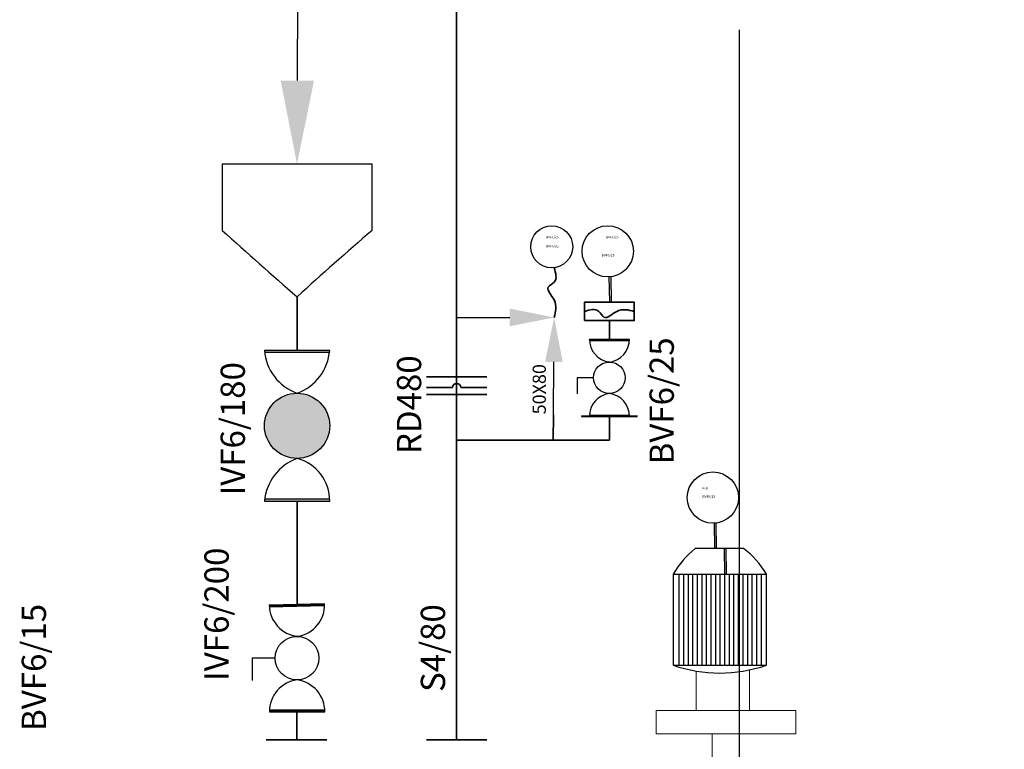
# Model space of a CAD drawing. Units: millimetres. Extents: x 353872 to 441597, y 126154 to 187356.
# Tile 12 of 28: x 391300 to 395281, y 149281 to 152234. Entities that reach past the tile are written whole.
import ezdxf

# ---------------------------------------------------------------- set-up
doc = ezdxf.new("R2010")
doc.units = ezdxf.units.MM
for name, color, linetype, lineweight in [('A-ANNO-DIMS', 2, 'Continuous', 18), ('P-ANNO-TEXT', 7, 'Continuous', 25), ('P-INST', 6, 'Continuous', 25), ('P-INST-SIGN', 4, 'Continuous', 18), ('P-PIPE', 3, 'Continuous', 35), ('P-PIPE-FITT', 6, 'Continuous', 25), ('P-SYMB-PATT', 8, 'Continuous', 13), ('P-VALV', 2, 'Continuous', 25)]:
    doc.layers.add(name, color=color, linetype=linetype, lineweight=lineweight)
doc.layers.add('AC-UINT', color=2, linetype='Continuous')
doc.styles.get("Standard").update_dxf_attribs({"font": 'arial.ttf'})
doc.dimstyles.get("Standard").update_dxf_attribs({"dimtxt": 0.18, "dimasz": 0.18, "dimexe": 0.18, "dimexo": 0.0625, "dimgap": 0.09, "dimtad": 0, "dimtih": 1, "dimtoh": 1, "dimdec": 4, "dimzin": 0, "dimdsep": 46, "dimtxsty": 'Standard', "dimcen": 0.09, "dimadec": 0, "dimazin": 0, "dimtfac": 1, "dimtdec": 4, "dimtofl": 0, "dimtmove": 0, "dimatfit": 3, "dimfxl": 1, "dimtolj": 1, "dimtzin": 0, "dimarcsym": 0})

# ---------------------------------------------------------------- blocks, each defined once
blk = doc.blocks.new('DFSG')
at = {"layer": 'AC-UINT', "ltscale": 3}
blk.add_line((94.3237, -27.1601), (94.091, -27.1601), dxfattribs=at)
blk.add_solid([(94.091, -27.1214), (94.0909, -27.1989), (93.8965, -27.1598)], dxfattribs=at)
blk = doc.blocks.new('VALVE-C')
for points in [[(0, 2.6), (0, 0), (224, 0), (224, 3.5)], [(0, 2.5), (0, 2.5), (221.5, 2.5), (224, 2.5)], [(0.1, 5.1), (224, 5.1)], [(0.2, 7.8), (223.9, 7.8)]]:
    blk.add_lwpolyline(points)
for centre, radius, start, end in [((128.5, 1.3), 128.5, 97.3612, 180.5798), ((96.1, 1.7), 128, 359.2193, 82.8397)]:
    blk.add_arc(centre, radius, start, end)
blk = doc.blocks.new('VALVE-K')
for points in [[(0, 90.9), (0, 92.8), (161.5, 92.8), (161.5, 90.3)], [(0, 91), (1.8, 91), (159.7, 91), (161.6, 91)], [(0, 89.1), (161.5, 89.2)], [(0.1, 87.2), (161.5, 87.2)]]:
    blk.add_lwpolyline(points)
for centre, radius, start, end in [((92.6, 91.9), 92.6, 179.4202, 262.6388), ((69.3, 91.6), 92.3, 277.1603, 0.7807)]:
    blk.add_arc(centre, radius, start, end)
blk = doc.blocks.new('VALVE-L')
for points in [[(0, 9.1), (263.6, 9)], [(0, 0), (263.8, 0), (263.8, 3)]]:
    blk.add_lwpolyline(points)
for centre, radius, start, end in [((204.3, -18.8), 205.1, 110.6617, 174.7476), ((86.2, 1.5), 177.6, 359.5088, 75.082)]:
    blk.add_arc(centre, radius, start, end)
blk = doc.blocks.new('VALVE-N')
for points in [[(263.8, 173.2), (0, 173.2)], [(262.9, 164.1), (0.9, 164.1)]]:
    blk.add_lwpolyline(points)
for centre, radius, start, end in [((199, 187.9), 199.6, 184.2463, 250.3444), ((63.7, 188.8), 200.7, 289.8639, 355.5453)]:
    blk.add_arc(centre, radius, start, end)
blk = doc.blocks.new('*D35')
at = {"layer": 'A-ANNO-DIMS', "color": 0, "lineweight": -2, "transparency": 16777216}
for p, q in [((394208.5, 152192.2), (394208.7, 152192.2)), ((394208.7, 152192.2), (394208.7, 149129.3)), ((394208.6, 144024.1), (394208.8, 144024.1)), ((394208.7, 144024), (394208.7, 144024.2))]:
    blk.add_line(p, q, dxfattribs=at)
at = {"layer": 'A-ANNO-DIMS', "color": 0, "transparency": 16777216}
blk.add_solid([(394208.7, 149129.3), (394208.7, 149129.3), (394208.7, 149129.2)], dxfattribs=at)
at = {"layer": 'Defpoints', "color": 0, "transparency": 16777216}
for p in [(394208.7, 149129.2), (394208.7, 144024.1)]:
    blk.add_point(p, dxfattribs=at)
at = {"layer": 'A-ANNO-DIMS', "color": 0, "transparency": 16777216, "insert": (394208.1, 152192.2), "char_height": 0.18, "attachment_point": 5}
blk.add_mtext('\\A1;R5105', dxfattribs=at)

msp = doc.modelspace()

# ---------------------------------------------------------------- hatches: boundary and pattern name
at = {"layer": 'P-SYMB-PATT'}
h = msp.add_hatch(color=256, dxfattribs=at)
h.dxf.hatch_style = 1
h.paths.add_polyline_path([(392553.56, 150895.47), (392289.77, 150895.47, 0.0114102), (392290.65, 150886.4), (392552.65, 150886.4, 0.0113502)])
h.paths.add_polyline_path([(392553.41, 150294.39), (392290.81, 150294.4, 0.0111203), (392289.77, 150285.34), (392553.56, 150285.34), (392553.56, 150288.39, 0.0084492)])
h = msp.add_hatch(color=256, dxfattribs=at)
h.dxf.hatch_style = 1
h.paths.add_polyline_path([(392553.56, 150590.4, 1), (392289.77, 150590.4, 1)])

# ---------------------------------------------------------------- linework, layer by layer
at = {"layer": 'P-INST'}
for p, q in [((393682.5, 151193.96), (393684.29, 151090.53)), ((393689.56, 151194.08), (393691.36, 151090.66)), ((394107.85, 150197.48), (394109.64, 150094.05)), ((394114.91, 150197.6), (394116.7, 150094.18)), ((394148.1, 150094.05), (394149.89, 149990.63)), ((394155.16, 150094.18), (394156.95, 149990.75)), ((393942.13, 149990.63), (394319.06, 149990.63)), ((393965.47, 149990.63), (393965.47, 149621.79)), ((393983.92, 149990.63), (393983.92, 149621.79)), ((394002.36, 149990.63), (394002.36, 149621.79)), ((394020.8, 149990.63), (394020.8, 149621.79)), ((394039.24, 149990.63), (394039.24, 149621.79)), ((394057.68, 149990.63), (394057.68, 149621.79)), ((394076.12, 149990.63), (394076.12, 149621.79)), ((394094.56, 149990.63), (394094.56, 149621.79)), ((394113.01, 149990.63), (394113.01, 149621.79)), ((394131.45, 149990.63), (394131.45, 149621.79)), ((394149.89, 149990.63), (394149.89, 149621.79)), ((394168.33, 149990.63), (394168.33, 149621.79)), ((394186.77, 149990.63), (394186.77, 149621.79)), ((394205.21, 149990.63), (394205.21, 149621.79)), ((394223.66, 149990.63), (394223.66, 149621.79)), ((394242.1, 149990.63), (394242.1, 149621.79)), ((394260.54, 149990.63), (394260.54, 149621.79)), ((394278.98, 149990.63), (394278.98, 149621.79)), ((394297.42, 149990.63), (394297.42, 149621.79))]:
    msp.add_line(p, q, dxfattribs=at)
for points in [[(392724.69, 151380.68), (392724.69, 151649.05), (392118.64, 151649.05), (392118.64, 151380.68)], [(394226.7, 150094.05), (394031.47, 150094.05)], [(393942.13, 149990.63), (393942.13, 149621.79), (394319.06, 149621.79), (394319.06, 149990.63)]]:
    msp.add_lwpolyline(points, dxfattribs=at)
for centre, radius in [((393451.3, 151314.58), 84.94), ((393677.68, 151296.37), 103.68), ((394103.03, 150299.89), 103.68)]:
    msp.add_circle(centre, radius, dxfattribs=at)
for centre, radius, start, end in [((415520.45, 177499.23), 35068.84, 228.140152, 228.801495), ((403079.21, 139383.76), 15847.46, 130.797418, 132.260935), ((394280.7, 149788.49), 394.31, 129.20292, 149.16161), ((394019.96, 149816.48), 346.11, 30.20977, 53.32091), ((394130.6, 150164.29), 574.31, 250.84308, 289.15692)]:
    msp.add_arc(centre, radius, start, end, dxfattribs=at)
at = {"layer": 'P-INST-SIGN'}
for p, q in [((394035.04, 149621.79), (394035.04, 149622.65)), ((394035.04, 149437.76), (394035.04, 149597.99)), ((394251.52, 149621.79), (394251.52, 149622.65)), ((394251.52, 149437.76), (394251.52, 149602.86)), ((394099.49, 149129.17), (394099.49, 149343.39)), ((394208.72, 149129.17), (394208.72, 149343.39))]:
    msp.add_line(p, q, dxfattribs=at)
msp.add_lwpolyline([(393873.52, 149343.39), (394437.89, 149343.39), (394437.89, 149437.76), (393873.52, 149437.76)], close=True, dxfattribs=at)
at = {"layer": 'P-PIPE'}
for p, q in [((392421.66, 151112.3), (392421.66, 150895.47)), ((393684.29, 150941.28), (393684.29, 151015.78)), ((393189.09, 150787.98), (392944.33, 150787.98)), ((393050.08, 150745.27), (392944.33, 150745.27)), ((393189.09, 150717.22), (392944.33, 150717.22)), ((393189.09, 150745.27), (393083.34, 150745.27)), ((393457.91, 150634.07), (393457, 150531.6)), ((393684.3, 150531.6), (393684.3, 150628.25)), ((393066.71, 150531.6), (393684.3, 150531.6)), ((392421.66, 150285.34), (392421.66, 149867.25)), ((392420.41, 149433.14), (392420.41, 149319.73)), ((392542.13, 149319.73), (392297.37, 149319.73)), ((393189.09, 149319.73), (392944.33, 149319.73))]:
    msp.add_line(p, q, dxfattribs=at)
msp.add_lwpolyline([(393066.71, 149319.73), (393066.71, 175399.89), (426420.76, 175399.89)], dxfattribs=at)
msp.add_lwpolyline([(393583.43, 151015.78), (393785.15, 151015.78), (393785.15, 151090.53), (393583.43, 151090.53)], close=True, dxfattribs=at)
msp.add_arc((393066.71, 150745.27), 16.63, 0, 180, dxfattribs=at)
for points in [[(393461.04, 151230.2), (393467.62, 151208.1), (393477.7, 151174.21), (393418.48, 151148.49), (393478.1, 151094.54), (393467.2, 151052.09), (393461.13, 151028.48)], [(393583.43, 151053.16), (393605.53, 151059.73), (393639.42, 151069.82), (393665.15, 151010.59), (393719.09, 151070.21), (393761.54, 151059.31), (393785.15, 151053.25)]]:
    msp.add_open_spline(points, degree=3, knots=[0, 0, 0, 0, 58.5959847, 89.8481435, 146.598413, 217.7037752, 217.7037752, 217.7037752, 217.7037752], dxfattribs=at)
at = {"layer": 'P-VALV'}
for points in [[(393620.41, 150784.76), (393553.75, 150784.76), (393553.75, 150719.31)], [(393572.27, 150630.85), (393572.27, 150628.25), (393796.3, 150628.25), (393796.3, 150631.74)], [(393603.55, 150631.94), (393765.04, 150631.91)], [(393603.63, 150633.85), (393764.97, 150633.89)], [(393572.27, 150630.79), (393572.27, 150630.79), (393793.79, 150630.76), (393796.3, 150630.76)], [(392333.08, 149650.19), (392240.63, 149650.19), (392240.63, 149559.43)]]:
    msp.add_lwpolyline(points, dxfattribs=at)
for centre, radius in [((393684.08, 150784.76), 63.66), ((392421.66, 150590.4), 131.9), ((392421.37, 149650.19), 88.29)]:
    msp.add_circle(centre, radius, dxfattribs=at)
for centre, radius, start, end in [((393696.16, 150629.19), 92.65, 97.36123, 180.57985), ((393672.79, 150629.51), 92.28, 359.21925, 82.83967)]:
    msp.add_arc(centre, radius, start, end, dxfattribs=at)

# ---------------------------------------------------------------- block references
at = {"layer": 'P-PIPE-FITT'}
for p, xscale, yscale, zscale, rotation in [((344986.64, -11465.79), 1737.899325704125, 1737.899325704125, 1737.899325704125, 89.91781771039466), ((480142.34, 125888.34), 923.3484342094463, 923.3484342094463, 923.3484342094463, 179.9589088552121), ((369155.52, 237947.38), -923.3484342094463, 923.3484342094465, 923.3484342094465, 89.49023455319704)]:
    msp.add_blockref('DFSG', p, dxfattribs=dict(at, xscale=xscale, yscale=yscale, zscale=zscale, rotation=rotation))
at = {"layer": 'P-VALV'}
for name, p in [('VALVE-K', (393603.52, 150848.46)), ('VALVE-N', (392289.77, 150722.3)), ('VALVE-L', (392289.77, 150285.34)), ('VALVE-C', (392309.65, 149433.14))]:
    msp.add_blockref(name, p, dxfattribs=at)
at = {"layer": 'P-VALV', "rotation": 181.3019170023694}
msp.add_blockref('VALVE-C', (392533.19, 149869.79), dxfattribs=at)

# ---------------------------------------------------------------- texts
at = {"layer": 'P-ANNO-TEXT'}
for s, p in [('BVF6/25', (393428.05, 151349.06)), ('BVF6/25', (393670.61, 151349.06)), ('BVF6/25', (393428.05, 151312.49)), ('BVF6/25', (393653.24, 151275.3)), ('K-0', (394060.7, 150332.79)), ('BVF6/25', (394060.7, 150298.83))]:
    msp.add_text(s, height=9.835, dxfattribs=at).set_placement(p)
for s, height, p in [('BVF6/25', 98.09, (393944.92, 150434.16)), ('IVF6/180', 98.09, (392210.83, 150308.53)), ('RD480', 98.09, (392923.49, 150475.6)), ('50X80', 53.38, (393427.61, 150636.66)), ('IVF6/200', 98.09, (392145.1, 149558)), ('BVF6/15', 98.09, (391406.52, 149355.66)), ('S4/80', 98.09, (393019.96, 149513.45))]:
    msp.add_text(s, height=height, rotation=90, dxfattribs=at).set_placement(p)

# ---------------------------------------------------------------- dimensions: what is measured, and where the dimension line sits
at = {"layer": 'A-ANNO-DIMS'}
dim = msp.add_radius_dim(center=(394208.72, 144024.11), mpoint=(394208.7, 149129.17), dimstyle='Standard', override={"dimdec": 0, "dimlfac": 1, "dimrnd": 0, "dimzin": 0, "dimdsep": 46, "dimlunit": 2}, dxfattribs=at)
dim.commit()
dim.dimension.update_dxf_attribs({"geometry": '*D35', "text_midpoint": (394208.07, 152192.2), "dimtype": 164})

doc.saveas('drawing.dxf')
